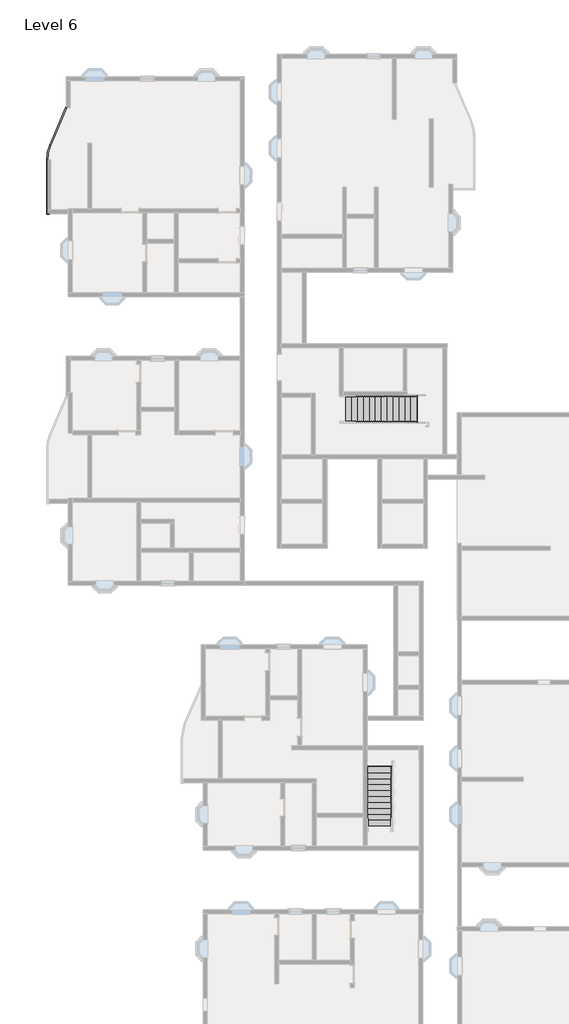
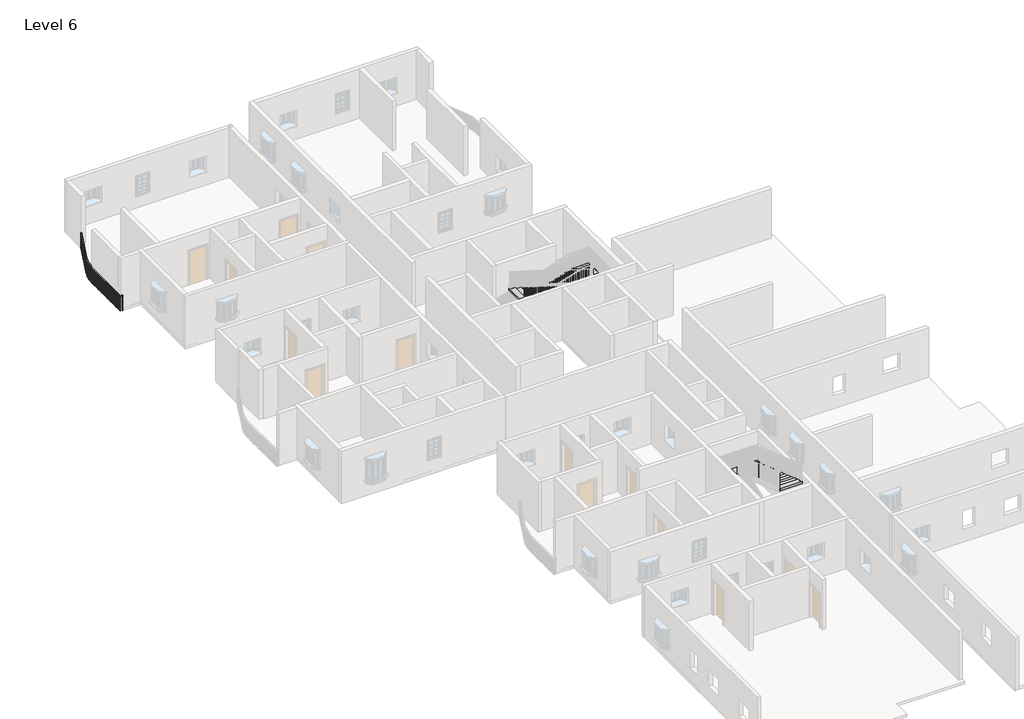
# One storey, part 12 of 14: 2 stair flights, 1 railing.
"""IFC4 building model written with IfcOpenShell, lengths in millimetres."""

from ifc_helpers import new_model, si_unit, frame, origin, place, context, project, spatial, polyline, circle_curve, outline, extrude, transform, mapped, element, save
from ifc_brep_helpers import plane_surface, cylinder_surface, revolved_surface, advanced_brep
from components import stair_flight_306d97fc, stair_flight_4df775fc

model = new_model("IFC4")

# Units and contexts
model_context = context("Model", 3, world=origin())
ifc_project = project(units=[si_unit("LENGTHUNIT", "METRE", prefix="MILLI")], contexts=[model_context])

# Site, building, storey
site = spatial("IfcSite", under=ifc_project)
building = spatial("IfcBuilding", under=site)
storey = spatial("IfcBuildingStorey", under=building, Name="Level 6", Elevation=15240.0)

# Railing
placement = place(None, origin())
element("IfcRailing", 1, ObjectType="Handrail - Rectangular", at=placement, inside=storey, context=model_context, shape_type="SolidModel", body=[
    advanced_brep(
    [(-19327.739878, 27355.8257339, 16154.4), (-19327.739878, 27355.8257339, 16103.6), (-19374.4383922, 27375.822953, 16103.6), (-19374.4383922, 27375.822953, 16154.4), (-20162.483418, 25406.4905323, 16154.4), (-20162.483418, 25406.4905323, 16103.6), (-20209.1819322, 25426.4877514, 16103.6), (-20209.1819322, 25426.4877514, 16154.4), (-20316.2891351, 24656.5948172, 16103.6), (-20316.2891351, 24656.5948172, 16154.4), (-20367.0891351, 24656.5948172, 16103.6), (-20367.0891351, 24656.5948172, 16154.4), (-20316.2891351, 21915.0583494, 16154.4), (-20316.2891351, 21915.0583494, 16103.6), (-20367.0891351, 21864.2583494, 16103.6), (-20367.0891351, 21864.2583494, 16154.4), (-20240.0891351, 21915.0583494, 16154.4), (-20240.0891351, 21864.2583494, 16154.4), (-20240.0891351, 21864.2583494, 16103.6), (-20240.0891351, 21915.0583494, 16103.6)],
    [
        (0, 1),
        (1, 2),
        (2, 3),
        (3, 0),
        (0, 4),
        (4, 5),
        (5, 1),
        (5, 6),
        (6, 2),
        (6, 7),
        (7, 3),
        (7, 4),
        (8, 5, circle_curve(frame((-18411.2891351, 24656.5948172, 16103.6), z_axis=(0.0, 0.0, -1.0), x_axis=(-0.9192620907623792, 0.3936460446736121, 0.0)), 1905.0)),
        (4, 9, circle_curve(frame((-18411.2891351, 24656.5948172, 16154.4), z_axis=(0.0, 0.0, 1.0), x_axis=(-0.9192620907623792, 0.3936460446736121, 0.0)), 1905.0)),
        (9, 8),
        (10, 6, circle_curve(frame((-18411.2891351, 24656.5948172, 16103.6), z_axis=(0.0, 0.0, -1.0), x_axis=(-0.9192620907623792, 0.3936460446736121, 0.0)), 1955.8)),
        (8, 10),
        (11, 7, circle_curve(frame((-18411.2891351, 24656.5948172, 16154.4), z_axis=(0.0, 0.0, -1.0), x_axis=(-0.9192620907623792, 0.3936460446736121, 0.0)), 1955.8)),
        (10, 11),
        (11, 9),
        (9, 12),
        (12, 13),
        (13, 8),
        (13, 14),
        (14, 10),
        (14, 15),
        (15, 11),
        (15, 12),
        (16, 17),
        (17, 18),
        (18, 19),
        (19, 16),
        (12, 16),
        (19, 13),
        (18, 14),
        (17, 15),
    ],
    [
        plane_surface(frame((-19351.0891351, 27365.8243434, 16154.4), z_axis=(0.3936460446736102, 0.91926209076238, 0.0), x_axis=(0.91926209076238, -0.3936460446736102, 0.0))),
        plane_surface(frame((-19327.739878, 27355.8257339, 16154.4), z_axis=(0.91926209076238, -0.3936460446736102, 0.0), x_axis=(-0.3936460446736102, -0.91926209076238, 0.0))),
        plane_surface(frame((-19327.739878, 27355.8257339, 16103.6), z_axis=(0.0, 0.0, -1.0), x_axis=(-0.3936460446736102, -0.91926209076238, 0.0))),
        plane_surface(frame((-19374.4383922, 27375.822953, 16103.6), z_axis=(-0.91926209076238, 0.3936460446736102, 0.0), x_axis=(-0.3936460446736102, -0.91926209076238, 0.0))),
        plane_surface(frame((-19374.4383922, 27375.822953, 16154.4), z_axis=(0.0, 0.0, 1.0), x_axis=(-0.3936460446736102, -0.91926209076238, 0.0))),
        revolved_surface(polyline([(-20162.48341800233, 25406.49053230323, 16154.4), (-20162.48341800233, 25406.49053230323, 16103.6)]), (-18411.2891351, 24656.5948172, 16154.4), (0.0, 0.0, 1.0)),
        plane_surface(frame((-18411.2891351, 24656.5948172, 16103.6), z_axis=(0.0, 0.0, -1.0), x_axis=(-0.9192620907623792, 0.3936460446736121, 0.0))),
        cylinder_surface(frame((-18411.2891351, 24656.5948172, 16154.4), z_axis=(0.0, 0.0, 1.0), x_axis=(-0.9192620907623792, 0.3936460446736121, 0.0)), 1955.8),
        plane_surface(frame((-18411.2891351, 24656.5948172, 16154.4), z_axis=(0.0, 0.0, 1.0), x_axis=(-0.9192620907623792, 0.3936460446736121, 0.0))),
        plane_surface(frame((-20316.2891351, 24656.5948172, 16154.4), z_axis=(1.0, 0.0, 0.0), x_axis=(0.0, -1.0, 0.0))),
        plane_surface(frame((-20316.2891351, 24656.5948172, 16103.6), z_axis=(0.0, 0.0, -1.0), x_axis=(0.0, -1.0, 0.0))),
        plane_surface(frame((-20367.0891351, 24656.5948172, 16103.6), z_axis=(-1.0, 0.0, 0.0), x_axis=(0.0, -1.0, 0.0))),
        plane_surface(frame((-20367.0891351, 24656.5948172, 16154.4), z_axis=(0.0, 0.0, 1.0), x_axis=(0.0, -1.0, 0.0))),
        plane_surface(frame((-20240.0891351, 21889.6583494, 16154.4), z_axis=(1.0, 0.0, 0.0), x_axis=(0.0, 1.0, 0.0))),
        plane_surface(frame((-20316.2891351, 21915.0583494, 16154.4), z_axis=(0.0, 1.0, 0.0), x_axis=(1.0, 0.0, 0.0))),
        plane_surface(frame((-20316.2891351, 21915.0583494, 16103.6), z_axis=(0.0, 0.0, -1.0), x_axis=(1.0, 0.0, 0.0))),
        plane_surface(frame((-20367.0891351, 21864.2583494, 16103.6), z_axis=(0.0, -1.0, 0.0), x_axis=(1.0, 0.0, 0.0))),
        plane_surface(frame((-20367.0891351, 21864.2583494, 16154.4), z_axis=(0.0, 0.0, 1.0), x_axis=(1.0, 0.0, 0.0))),
    ],
    [
        (0, [[1, 2, 3, 4]]),
        (1, [[-1, 5, 6, 7]]),
        (2, [[-2, -7, 8, 9]]),
        (3, [[-3, -9, 10, 11]]),
        (4, [[-4, -11, 12, -5]]),
        (5, [[13, -6, 14, 15]]),
        (6, [[16, -8, -13, 17]]),
        (7, [[18, -10, -16, 19]]),
        (8, [[-14, -12, -18, 20]]),
        (9, [[-15, 21, 22, 23]]),
        (10, [[-17, -23, 24, 25]]),
        (11, [[-19, -25, 26, 27]]),
        (12, [[-20, -27, 28, -21]]),
        (13, [[29, 30, 31, 32]]),
        (14, [[-22, 33, -32, 34]]),
        (15, [[-24, -34, -31, 35]]),
        (16, [[-26, -35, -30, 36]]),
        (17, [[-28, -36, -29, -33]]),
    ],
),
    extrude(outline(polyline([(-20351.2141351, 21922.9198172), (-20332.1641351, 21922.9198172), (-20332.1641351, 21903.8698172), (-20351.2141351, 21903.8698172), (-20351.2141351, 21922.9198172)])), frame((0.0, 0.0, 15240.0), z_axis=(0.0, 0.0, 1.0), x_axis=(1.0, 0.0, 0.0)), (0.0, 0.0, 1.0), 863.6),
    extrude(outline(polyline([(-20351.2141351, 22024.5198172), (-20332.1641351, 22024.5198172), (-20332.1641351, 22005.4698172), (-20351.2141351, 22005.4698172), (-20351.2141351, 22024.5198172)])), frame((0.0, 0.0, 15240.0), z_axis=(0.0, 0.0, 1.0), x_axis=(1.0, 0.0, 0.0)), (0.0, 0.0, 1.0), 863.6),
    extrude(outline(polyline([(-20351.2141351, 22126.1198172), (-20332.1641351, 22126.1198172), (-20332.1641351, 22107.0698172), (-20351.2141351, 22107.0698172), (-20351.2141351, 22126.1198172)])), frame((0.0, 0.0, 15240.0), z_axis=(0.0, 0.0, 1.0), x_axis=(1.0, 0.0, 0.0)), (0.0, 0.0, 1.0), 863.6),
    extrude(outline(polyline([(-20351.2141351, 22227.7198172), (-20332.1641351, 22227.7198172), (-20332.1641351, 22208.6698172), (-20351.2141351, 22208.6698172), (-20351.2141351, 22227.7198172)])), frame((0.0, 0.0, 15240.0), z_axis=(0.0, 0.0, 1.0), x_axis=(1.0, 0.0, 0.0)), (0.0, 0.0, 1.0), 863.6),
    extrude(outline(polyline([(-20351.2141351, 22329.3198172), (-20332.1641351, 22329.3198172), (-20332.1641351, 22310.2698172), (-20351.2141351, 22310.2698172), (-20351.2141351, 22329.3198172)])), frame((0.0, 0.0, 15240.0), z_axis=(0.0, 0.0, 1.0), x_axis=(1.0, 0.0, 0.0)), (0.0, 0.0, 1.0), 863.6),
    extrude(outline(polyline([(-20351.2141351, 22430.9198172), (-20332.1641351, 22430.9198172), (-20332.1641351, 22411.8698172), (-20351.2141351, 22411.8698172), (-20351.2141351, 22430.9198172)])), frame((0.0, 0.0, 15240.0), z_axis=(0.0, 0.0, 1.0), x_axis=(1.0, 0.0, 0.0)), (0.0, 0.0, 1.0), 863.6),
    extrude(outline(polyline([(-20351.2141351, 22532.5198172), (-20332.1641351, 22532.5198172), (-20332.1641351, 22513.4698172), (-20351.2141351, 22513.4698172), (-20351.2141351, 22532.5198172)])), frame((0.0, 0.0, 15240.0), z_axis=(0.0, 0.0, 1.0), x_axis=(1.0, 0.0, 0.0)), (0.0, 0.0, 1.0), 863.6),
    extrude(outline(polyline([(-20351.2141351, 22634.1198172), (-20332.1641351, 22634.1198172), (-20332.1641351, 22615.0698172), (-20351.2141351, 22615.0698172), (-20351.2141351, 22634.1198172)])), frame((0.0, 0.0, 15240.0), z_axis=(0.0, 0.0, 1.0), x_axis=(1.0, 0.0, 0.0)), (0.0, 0.0, 1.0), 863.6),
    extrude(outline(polyline([(-20351.2141351, 22735.7198172), (-20332.1641351, 22735.7198172), (-20332.1641351, 22716.6698172), (-20351.2141351, 22716.6698172), (-20351.2141351, 22735.7198172)])), frame((0.0, 0.0, 15240.0), z_axis=(0.0, 0.0, 1.0), x_axis=(1.0, 0.0, 0.0)), (0.0, 0.0, 1.0), 863.6),
    extrude(outline(polyline([(-20351.2141351, 22837.3198172), (-20332.1641351, 22837.3198172), (-20332.1641351, 22818.2698172), (-20351.2141351, 22818.2698172), (-20351.2141351, 22837.3198172)])), frame((0.0, 0.0, 15240.0), z_axis=(0.0, 0.0, 1.0), x_axis=(1.0, 0.0, 0.0)), (0.0, 0.0, 1.0), 863.6),
    extrude(outline(polyline([(-20351.2141351, 22938.9198172), (-20332.1641351, 22938.9198172), (-20332.1641351, 22919.8698172), (-20351.2141351, 22919.8698172), (-20351.2141351, 22938.9198172)])), frame((0.0, 0.0, 15240.0), z_axis=(0.0, 0.0, 1.0), x_axis=(1.0, 0.0, 0.0)), (0.0, 0.0, 1.0), 863.6),
    extrude(outline(polyline([(-20351.2141351, 23040.5198172), (-20332.1641351, 23040.5198172), (-20332.1641351, 23021.4698172), (-20351.2141351, 23021.4698172), (-20351.2141351, 23040.5198172)])), frame((0.0, 0.0, 15240.0), z_axis=(0.0, 0.0, 1.0), x_axis=(1.0, 0.0, 0.0)), (0.0, 0.0, 1.0), 863.6),
    extrude(outline(polyline([(-20351.2141351, 23142.1198172), (-20332.1641351, 23142.1198172), (-20332.1641351, 23123.0698172), (-20351.2141351, 23123.0698172), (-20351.2141351, 23142.1198172)])), frame((0.0, 0.0, 15240.0), z_axis=(0.0, 0.0, 1.0), x_axis=(1.0, 0.0, 0.0)), (0.0, 0.0, 1.0), 863.6),
    extrude(outline(polyline([(-20351.2141351, 23243.7198172), (-20332.1641351, 23243.7198172), (-20332.1641351, 23224.6698172), (-20351.2141351, 23224.6698172), (-20351.2141351, 23243.7198172)])), frame((0.0, 0.0, 15240.0), z_axis=(0.0, 0.0, 1.0), x_axis=(1.0, 0.0, 0.0)), (0.0, 0.0, 1.0), 863.6),
    extrude(outline(polyline([(-20351.2141351, 23345.3198172), (-20332.1641351, 23345.3198172), (-20332.1641351, 23326.2698172), (-20351.2141351, 23326.2698172), (-20351.2141351, 23345.3198172)])), frame((0.0, 0.0, 15240.0), z_axis=(0.0, 0.0, 1.0), x_axis=(1.0, 0.0, 0.0)), (0.0, 0.0, 1.0), 863.6),
    extrude(outline(polyline([(-20351.2141351, 23446.9198172), (-20332.1641351, 23446.9198172), (-20332.1641351, 23427.8698172), (-20351.2141351, 23427.8698172), (-20351.2141351, 23446.9198172)])), frame((0.0, 0.0, 15240.0), z_axis=(0.0, 0.0, 1.0), x_axis=(1.0, 0.0, 0.0)), (0.0, 0.0, 1.0), 863.6),
    extrude(outline(polyline([(-20351.2141351, 23548.5198172), (-20332.1641351, 23548.5198172), (-20332.1641351, 23529.4698172), (-20351.2141351, 23529.4698172), (-20351.2141351, 23548.5198172)])), frame((0.0, 0.0, 15240.0), z_axis=(0.0, 0.0, 1.0), x_axis=(1.0, 0.0, 0.0)), (0.0, 0.0, 1.0), 863.6),
    extrude(outline(polyline([(-20351.2141351, 23650.1198172), (-20332.1641351, 23650.1198172), (-20332.1641351, 23631.0698172), (-20351.2141351, 23631.0698172), (-20351.2141351, 23650.1198172)])), frame((0.0, 0.0, 15240.0), z_axis=(0.0, 0.0, 1.0), x_axis=(1.0, 0.0, 0.0)), (0.0, 0.0, 1.0), 863.6),
    extrude(outline(polyline([(-20351.2141351, 23751.7198172), (-20332.1641351, 23751.7198172), (-20332.1641351, 23732.6698172), (-20351.2141351, 23732.6698172), (-20351.2141351, 23751.7198172)])), frame((0.0, 0.0, 15240.0), z_axis=(0.0, 0.0, 1.0), x_axis=(1.0, 0.0, 0.0)), (0.0, 0.0, 1.0), 863.6),
    extrude(outline(polyline([(-20351.2141351, 23853.3198172), (-20332.1641351, 23853.3198172), (-20332.1641351, 23834.2698172), (-20351.2141351, 23834.2698172), (-20351.2141351, 23853.3198172)])), frame((0.0, 0.0, 15240.0), z_axis=(0.0, 0.0, 1.0), x_axis=(1.0, 0.0, 0.0)), (0.0, 0.0, 1.0), 863.6),
    extrude(outline(polyline([(-20351.2141351, 23954.9198172), (-20332.1641351, 23954.9198172), (-20332.1641351, 23935.8698172), (-20351.2141351, 23935.8698172), (-20351.2141351, 23954.9198172)])), frame((0.0, 0.0, 15240.0), z_axis=(0.0, 0.0, 1.0), x_axis=(1.0, 0.0, 0.0)), (0.0, 0.0, 1.0), 863.6),
    extrude(outline(polyline([(-20351.2141351, 24056.5198172), (-20332.1641351, 24056.5198172), (-20332.1641351, 24037.4698172), (-20351.2141351, 24037.4698172), (-20351.2141351, 24056.5198172)])), frame((0.0, 0.0, 15240.0), z_axis=(0.0, 0.0, 1.0), x_axis=(1.0, 0.0, 0.0)), (0.0, 0.0, 1.0), 863.6),
    extrude(outline(polyline([(-20351.2141351, 24158.1198172), (-20332.1641351, 24158.1198172), (-20332.1641351, 24139.0698172), (-20351.2141351, 24139.0698172), (-20351.2141351, 24158.1198172)])), frame((0.0, 0.0, 15240.0), z_axis=(0.0, 0.0, 1.0), x_axis=(1.0, 0.0, 0.0)), (0.0, 0.0, 1.0), 863.6),
    extrude(outline(polyline([(-20351.2141351, 24259.7198172), (-20332.1641351, 24259.7198172), (-20332.1641351, 24240.6698172), (-20351.2141351, 24240.6698172), (-20351.2141351, 24259.7198172)])), frame((0.0, 0.0, 15240.0), z_axis=(0.0, 0.0, 1.0), x_axis=(1.0, 0.0, 0.0)), (0.0, 0.0, 1.0), 863.6),
    extrude(outline(polyline([(-20351.2141351, 24361.3198172), (-20332.1641351, 24361.3198172), (-20332.1641351, 24342.2698172), (-20351.2141351, 24342.2698172), (-20351.2141351, 24361.3198172)])), frame((0.0, 0.0, 15240.0), z_axis=(0.0, 0.0, 1.0), x_axis=(1.0, 0.0, 0.0)), (0.0, 0.0, 1.0), 863.6),
    extrude(outline(polyline([(-20351.2141351, 24462.9198172), (-20332.1641351, 24462.9198172), (-20332.1641351, 24443.8698172), (-20351.2141351, 24443.8698172), (-20351.2141351, 24462.9198172)])), frame((0.0, 0.0, 15240.0), z_axis=(0.0, 0.0, 1.0), x_axis=(1.0, 0.0, 0.0)), (0.0, 0.0, 1.0), 863.6),
    extrude(outline(polyline([(-20351.2141351, 24564.5198172), (-20332.1641351, 24564.5198172), (-20332.1641351, 24545.4698172), (-20351.2141351, 24545.4698172), (-20351.2141351, 24564.5198172)])), frame((0.0, 0.0, 15240.0), z_axis=(0.0, 0.0, 1.0), x_axis=(1.0, 0.0, 0.0)), (0.0, 0.0, 1.0), 863.6),
    extrude(outline(polyline([(-20349.6005818, 24736.2720848), (-20330.5630441, 24735.5831307), (-20331.2519982, 24716.545593), (-20350.289536, 24717.2345471), (-20349.6005818, 24736.2720848)])), frame((0.0, 0.0, 15240.0), z_axis=(0.0, 0.0, 1.0), x_axis=(1.0, 0.0, 0.0)), (0.0, 0.0, 1.0), 863.6),
    extrude(outline(polyline([(-20342.724955, 24838.1310534), (-20323.750023, 24836.4415402), (-20325.4395363, 24817.4666081), (-20344.4144683, 24819.1561214), (-20342.724955, 24838.1310534)])), frame((0.0, 0.0, 15240.0), z_axis=(0.0, 0.0, 1.0), x_axis=(1.0, 0.0, 0.0)), (0.0, 0.0, 1.0), 863.6),
    extrude(outline(polyline([(-20330.5003254, 24939.4872677), (-20311.6405491, 24936.8018743), (-20314.3259425, 24917.942098), (-20333.1857188, 24920.6274914), (-20330.5003254, 24939.4872677)])), frame((0.0, 0.0, 15240.0), z_axis=(0.0, 0.0, 1.0), x_axis=(1.0, 0.0, 0.0)), (0.0, 0.0, 1.0), 863.6),
    extrude(outline(polyline([(-20312.9605484, 25040.0600272), (-20294.2681589, 25036.3861907), (-20297.9419954, 25017.6938012), (-20316.6343849, 25021.3676377), (-20312.9605484, 25040.0600272)])), frame((0.0, 0.0, 15240.0), z_axis=(0.0, 0.0, 1.0), x_axis=(1.0, 0.0, 0.0)), (0.0, 0.0, 1.0), 863.6),
    extrude(outline(polyline([(-20290.1541995, 25139.5708014), (-20271.6809643, 25134.9186963), (-20276.3330693, 25116.4454611), (-20294.8063045, 25121.0975662), (-20290.1541995, 25139.5708014)])), frame((0.0, 0.0, 15240.0), z_axis=(0.0, 0.0, 1.0), x_axis=(1.0, 0.0, 0.0)), (0.0, 0.0, 1.0), 863.6),
    extrude(outline(polyline([(-20262.1444395, 25237.7440008), (-20243.9415192, 25232.1265109), (-20249.5590091, 25213.9235906), (-20267.7619294, 25219.5410805), (-20262.1444395, 25237.7440008)])), frame((0.0, 0.0, 15240.0), z_axis=(0.0, 0.0, 1.0), x_axis=(1.0, 0.0, 0.0)), (0.0, 0.0, 1.0), 863.6),
    extrude(outline(polyline([(-20229.0088399, 25334.3077402), (-20211.1266465, 25327.7404228), (-20217.693964, 25309.8582293), (-20235.5761574, 25316.4255468), (-20229.0088399, 25334.3077402)])), frame((0.0, 0.0, 15240.0), z_axis=(0.0, 0.0, 1.0), x_axis=(1.0, 0.0, 0.0)), (0.0, 0.0, 1.0), 863.6),
    extrude(outline(polyline([(-20155.9843907, 25510.389225), (-20138.4724479, 25502.8902678), (-20145.9714051, 25485.378325), (-20163.4833479, 25492.8772822), (-20155.9843907, 25510.389225)])), frame((0.0, 0.0, 15240.0), z_axis=(0.0, 0.0, 1.0), x_axis=(1.0, 0.0, 0.0)), (0.0, 0.0, 1.0), 863.6),
    extrude(outline(polyline([(-20115.9899526, 25603.7862534), (-20098.4780098, 25596.2872963), (-20105.9769669, 25578.7753534), (-20123.4889098, 25586.2743106), (-20115.9899526, 25603.7862534)])), frame((0.0, 0.0, 15240.0), z_axis=(0.0, 0.0, 1.0), x_axis=(1.0, 0.0, 0.0)), (0.0, 0.0, 1.0), 863.6),
    extrude(outline(polyline([(-20075.9955145, 25697.1832818), (-20058.4835716, 25689.6843247), (-20065.9825288, 25672.1723818), (-20083.4944716, 25679.671339), (-20075.9955145, 25697.1832818)])), frame((0.0, 0.0, 15240.0), z_axis=(0.0, 0.0, 1.0), x_axis=(1.0, 0.0, 0.0)), (0.0, 0.0, 1.0), 863.6),
    extrude(outline(polyline([(-20036.0010763, 25790.5803103), (-20018.4891335, 25783.0813531), (-20025.9880906, 25765.5694103), (-20043.5000335, 25773.0683674), (-20036.0010763, 25790.5803103)])), frame((0.0, 0.0, 15240.0), z_axis=(0.0, 0.0, 1.0), x_axis=(1.0, 0.0, 0.0)), (0.0, 0.0, 1.0), 863.6),
    extrude(outline(polyline([(-19996.0066382, 25883.9773387), (-19978.4946954, 25876.4783815), (-19985.9936525, 25858.9664387), (-20003.5055953, 25866.4653958), (-19996.0066382, 25883.9773387)])), frame((0.0, 0.0, 15240.0), z_axis=(0.0, 0.0, 1.0), x_axis=(1.0, 0.0, 0.0)), (0.0, 0.0, 1.0), 863.6),
    extrude(outline(polyline([(-19956.0122, 25977.3743671), (-19938.5002572, 25969.8754099), (-19945.9992144, 25952.3634671), (-19963.5111572, 25959.8624243), (-19956.0122, 25977.3743671)])), frame((0.0, 0.0, 15240.0), z_axis=(0.0, 0.0, 1.0), x_axis=(1.0, 0.0, 0.0)), (0.0, 0.0, 1.0), 863.6),
    extrude(outline(polyline([(-19916.0177619, 26070.7713955), (-19898.5058191, 26063.2724384), (-19906.0047762, 26045.7604955), (-19923.5167191, 26053.2594527), (-19916.0177619, 26070.7713955)])), frame((0.0, 0.0, 15240.0), z_axis=(0.0, 0.0, 1.0), x_axis=(1.0, 0.0, 0.0)), (0.0, 0.0, 1.0), 863.6),
    extrude(outline(polyline([(-19876.0233238, 26164.1684239), (-19858.5113809, 26156.6694668), (-19866.0103381, 26139.157524), (-19883.5222809, 26146.6564811), (-19876.0233238, 26164.1684239)])), frame((0.0, 0.0, 15240.0), z_axis=(0.0, 0.0, 1.0), x_axis=(1.0, 0.0, 0.0)), (0.0, 0.0, 1.0), 863.6),
    extrude(outline(polyline([(-19836.0288856, 26257.5654524), (-19818.5169428, 26250.0664952), (-19826.0159, 26232.5545524), (-19843.5278428, 26240.0535095), (-19836.0288856, 26257.5654524)])), frame((0.0, 0.0, 15240.0), z_axis=(0.0, 0.0, 1.0), x_axis=(1.0, 0.0, 0.0)), (0.0, 0.0, 1.0), 863.6),
    extrude(outline(polyline([(-19796.0344475, 26350.9624808), (-19778.5225047, 26343.4635236), (-19786.0214618, 26325.9515808), (-19803.5334046, 26333.450538), (-19796.0344475, 26350.9624808)])), frame((0.0, 0.0, 15240.0), z_axis=(0.0, 0.0, 1.0), x_axis=(1.0, 0.0, 0.0)), (0.0, 0.0, 1.0), 863.6),
    extrude(outline(polyline([(-19756.0400094, 26444.3595092), (-19738.5280665, 26436.860552), (-19746.0270237, 26419.3486092), (-19763.5389665, 26426.8475664), (-19756.0400094, 26444.3595092)])), frame((0.0, 0.0, 15240.0), z_axis=(0.0, 0.0, 1.0), x_axis=(1.0, 0.0, 0.0)), (0.0, 0.0, 1.0), 863.6),
    extrude(outline(polyline([(-19716.0455712, 26537.7565376), (-19698.5336284, 26530.2575805), (-19706.0325855, 26512.7456376), (-19723.5445284, 26520.2445948), (-19716.0455712, 26537.7565376)])), frame((0.0, 0.0, 15240.0), z_axis=(0.0, 0.0, 1.0), x_axis=(1.0, 0.0, 0.0)), (0.0, 0.0, 1.0), 863.6),
    extrude(outline(polyline([(-19676.0511331, 26631.153566), (-19658.5391902, 26623.6546089), (-19666.0381474, 26606.1426661), (-19683.5500902, 26613.6416232), (-19676.0511331, 26631.153566)])), frame((0.0, 0.0, 15240.0), z_axis=(0.0, 0.0, 1.0), x_axis=(1.0, 0.0, 0.0)), (0.0, 0.0, 1.0), 863.6),
    extrude(outline(polyline([(-19636.0566949, 26724.5505945), (-19618.5447521, 26717.0516373), (-19626.0437093, 26699.5396945), (-19643.5556521, 26707.0386516), (-19636.0566949, 26724.5505945)])), frame((0.0, 0.0, 15240.0), z_axis=(0.0, 0.0, 1.0), x_axis=(1.0, 0.0, 0.0)), (0.0, 0.0, 1.0), 863.6),
    extrude(outline(polyline([(-19596.0622568, 26817.9476229), (-19578.550314, 26810.4486657), (-19586.0492711, 26792.9367229), (-19603.561214, 26800.4356801), (-19596.0622568, 26817.9476229)])), frame((0.0, 0.0, 15240.0), z_axis=(0.0, 0.0, 1.0), x_axis=(1.0, 0.0, 0.0)), (0.0, 0.0, 1.0), 863.6),
    extrude(outline(polyline([(-19556.0678187, 26911.3446513), (-19538.5558758, 26903.8456942), (-19546.054833, 26886.3337513), (-19563.5667758, 26893.8327085), (-19556.0678187, 26911.3446513)])), frame((0.0, 0.0, 15240.0), z_axis=(0.0, 0.0, 1.0), x_axis=(1.0, 0.0, 0.0)), (0.0, 0.0, 1.0), 863.6),
    extrude(outline(polyline([(-19516.0733805, 27004.7416797), (-19498.5614377, 26997.2427226), (-19506.0603948, 26979.7307797), (-19523.5723377, 26987.2297369), (-19516.0733805, 27004.7416797)])), frame((0.0, 0.0, 15240.0), z_axis=(0.0, 0.0, 1.0), x_axis=(1.0, 0.0, 0.0)), (0.0, 0.0, 1.0), 863.6),
    extrude(outline(polyline([(-19476.0789424, 27098.1387082), (-19458.5669996, 27090.639751), (-19466.0659567, 27073.1278082), (-19483.5778995, 27080.6267653), (-19476.0789424, 27098.1387082)])), frame((0.0, 0.0, 15240.0), z_axis=(0.0, 0.0, 1.0), x_axis=(1.0, 0.0, 0.0)), (0.0, 0.0, 1.0), 863.6),
    extrude(outline(polyline([(-19436.0845042, 27191.5357366), (-19418.5725614, 27184.0367794), (-19426.0715186, 27166.5248366), (-19443.5834614, 27174.0237937), (-19436.0845042, 27191.5357366)])), frame((0.0, 0.0, 15240.0), z_axis=(0.0, 0.0, 1.0), x_axis=(1.0, 0.0, 0.0)), (0.0, 0.0, 1.0), 863.6),
    extrude(outline(polyline([(-19396.0900661, 27284.932765), (-19378.5781233, 27277.4338078), (-19386.0770804, 27259.921865), (-19403.5890233, 27267.4208222), (-19396.0900661, 27284.932765)])), frame((0.0, 0.0, 15240.0), z_axis=(0.0, 0.0, 1.0), x_axis=(1.0, 0.0, 0.0)), (0.0, 0.0, 1.0), 863.6),
    extrude(outline(polyline([(-20351.2141351, 21899.1833494), (-20332.1641351, 21899.1833494), (-20332.1641351, 21880.1333494), (-20351.2141351, 21880.1333494), (-20351.2141351, 21899.1833494)])), frame((0.0, 0.0, 15240.0), z_axis=(0.0, 0.0, 1.0), x_axis=(1.0, 0.0, 0.0)), (0.0, 0.0, 1.0), 863.6),
    extrude(outline(polyline([(-20351.2141351, 24666.1198172), (-20332.1641351, 24666.1198172), (-20332.1641351, 24647.0698172), (-20351.2141351, 24647.0698172), (-20351.2141351, 24666.1198172)])), frame((0.0, 0.0, 15240.0), z_axis=(0.0, 0.0, 1.0), x_axis=(1.0, 0.0, 0.0)), (0.0, 0.0, 1.0), 863.6),
    extrude(outline(polyline([(-20190.839168, 25428.9945919), (-20173.3272251, 25421.4956347), (-20180.8261823, 25403.9836919), (-20198.3381251, 25411.482649), (-20190.839168, 25428.9945919)])), frame((0.0, 0.0, 15240.0), z_axis=(0.0, 0.0, 1.0), x_axis=(1.0, 0.0, 0.0)), (0.0, 0.0, 1.0), 863.6),
    extrude(outline(polyline([(-20259.1391351, 21880.1333494), (-20259.1391351, 21899.1833494), (-20240.0891351, 21899.1833494), (-20240.0891351, 21880.1333494), (-20259.1391351, 21880.1333494)])), frame((0.0, 0.0, 15240.0), z_axis=(0.0, 0.0, 1.0), x_axis=(1.0, 0.0, 0.0)), (0.0, 0.0, 1.0), 863.6),
    extrude(outline(polyline([(-19359.8451065, 27369.573822), (-19342.3331637, 27362.0748648), (-19349.8321209, 27344.562922), (-19367.3440637, 27352.0618792), (-19359.8451065, 27369.573822)])), frame((0.0, 0.0, 15240.0), z_axis=(0.0, 0.0, 1.0), x_axis=(1.0, 0.0, 0.0)), (0.0, 0.0, 1.0), 863.6),
])

# Stair flights
stair_flight_shape = stair_flight_306d97fc(model_context)
element("IfcStairFlight", 2, ObjectType="2\" Tread 1\" Nosing 1/4\" Riser", at=placement, inside=storey, context=model_context, shape_type="MappedRepresentation", body=[
    mapped(stair_flight_shape, transform((0.0, 0.0, 0.0), x_axis=(1.0, 0.0, 0.0), y_axis=(0.0, 1.0, 0.0), z_axis=(0.0, 0.0, 1.0))),
])
stair_flight_2_shape = stair_flight_4df775fc(model_context)
element("IfcStairFlight", 3, ObjectType="2\" Tread 1\" Nosing 1/4\" Riser", at=placement, inside=storey, context=model_context, shape_type="MappedRepresentation", body=[
    mapped(stair_flight_2_shape, transform((0.0, 0.0, 0.0), x_axis=(1.0, 0.0, 0.0), y_axis=(0.0, 1.0, 0.0), z_axis=(0.0, 0.0, 1.0))),
])

save(model, "model.ifc")

# Revit data of these elements
# Type "Handrail - Rectangular"
#   Assembly Code = "C2010400"
#   built-in parameter 1008612 = 0.0416667 (stored number, unit not read)
#   built-in parameter 1008611 = 0.0416667 (stored number, unit not read)
#   built-in parameter 1008609 = 0.333333 (stored number, unit not read)
#   built-in parameter 1008604 = 0.166667 (stored number, unit not read)
#   built-in parameter 1008603 = 0.166667 (stored number, unit not read)
#   Railing Height = 3' - 0"
#   built-in parameter 1008630 = 2
#   built-in parameter 1008610 = 2
#   built-in parameter 1008618 = Baluster - Square : 3/4"
# Element 1 (IfcRailing, "Handrail - Rectangular")
#   Phase Created = New Construction
# Elements 2, 3 (IfcStairFlight, "2\" Tread 1\" Nosing 1/4\" Riser")
#   Phase Created = New Construction
